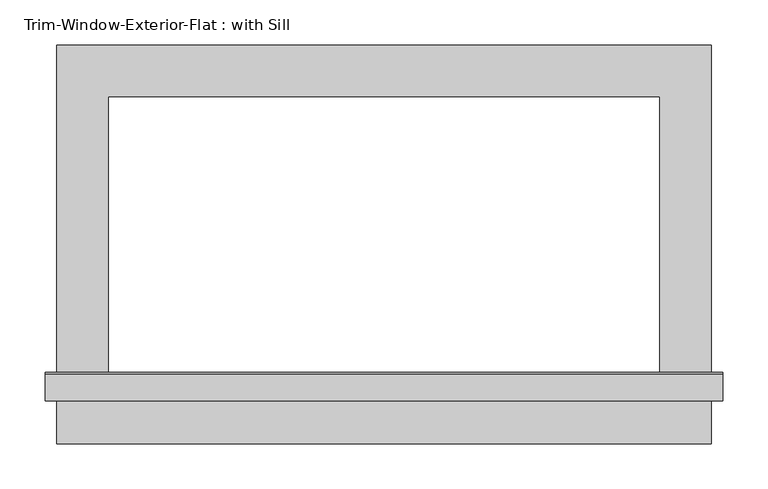
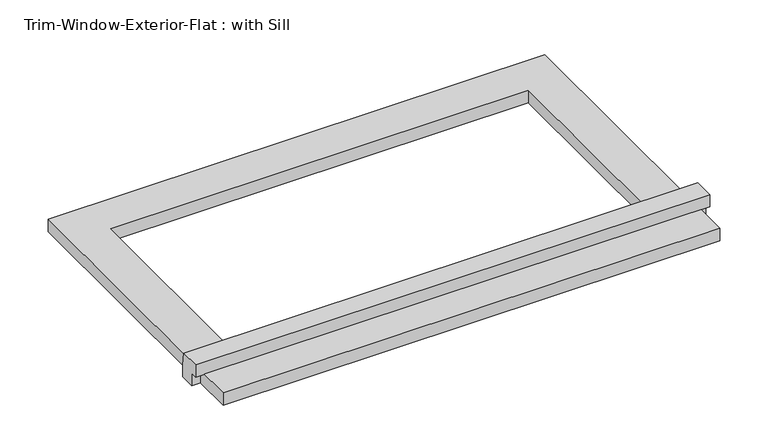
"""IFC4 building model written with IfcOpenShell, lengths in millimetres: proxy geometry, Trim-Window-Exterior-Flat : with Sill."""

from ifc_helpers import new_model, si_unit, frame, origin, origin_with_axes, place, context, project, spatial, polyline, outline, extrude, source, transform, mapped, element, save


def trim_window_exterior_flat_with_sill_281d40e2(model_context):
    return source(origin(), model_context, "Body", "SweptSolid", [
        extrude(outline(polyline([(361.95, -326.9823709), (361.95, -384.1323709), (-361.95, -384.1323709), (-361.95, -326.9823709), (361.95, -326.9823709)])), origin_with_axes(), (0.0, 0.0, 1.0), 19.05),
        extrude(outline(polyline([(-336.55, 38.1), (-307.2580645, 38.1), (-304.8, 19.05), (-304.8, 0.0), (-326.9823709, 0.0), (-326.9823709, 19.05), (-336.55, 19.05), (-336.55, 38.1)])), frame((-374.65, 0.0, 0.0), z_axis=(1.0, 0.0, 0.0), x_axis=(0.0, 1.0, 0.0)), (0.0, 0.0, 1.0), 749.3),
        extrude(outline(polyline([(-361.95, 57.15), (361.95, 57.15), (361.95, -304.8), (304.8, -304.8), (304.8, 0.0), (-304.8, 0.0), (-304.8, -304.8), (-361.95, -304.8), (-361.95, 57.15)])), origin_with_axes(), (0.0, 0.0, 1.0), 19.05),
    ])


if __name__ == "__main__":
    model = new_model("IFC4")
    model_context = context("Model", 3, world=origin())
    ifc_project = project(units=[si_unit("LENGTHUNIT", "METRE", prefix="MILLI")], contexts=[model_context])
    site = spatial("IfcSite", under=ifc_project)
    building = spatial("IfcBuilding", under=site)
    placement = place(None, origin())
    trim_window_exterior_flat_with_sill_shape = trim_window_exterior_flat_with_sill_281d40e2(model_context)
    element("IfcBuildingElementProxy", 1, Name="Trim-Window-Exterior-Flat : with Sill", ObjectType="Trim-Window-Exterior-Flat : with Sill", at=placement, inside=building, context=model_context, shape_type="MappedRepresentation", body=[
        mapped(trim_window_exterior_flat_with_sill_shape, transform((0.0, 0.0, 0.0), x_axis=(1.0, 0.0, 0.0), y_axis=(0.0, 1.0, 0.0), z_axis=(0.0, 0.0, 1.0))),
    ])
    save(model, "model.ifc")

# Revit data of these elements
# Type "Trim-Window-Exterior-Flat : with Sill"
#   Trim Width = 0' - 2 1/4"
#   Trim Thickness_Picture Frame = 0' - 1 1/4"
#   Trim Thickness_with Sill = 0' - 0 3/4"
#   Sill Thickness = 0' - 1 1/4"
#   Opening Width [instance default] = 2' - 0"
#   Opening Height [instance default] = 3' - 0"
#   Default Elevation = 4' - 0"
#   Sill = yes
#   Picture Frame = no
#   Trim Material [instance default] = none
# Element 1 (IfcBuildingElementProxy, "Trim-Window-Exterior-Flat : with Sill")
#   Opening Height = 1' - 0"
#   Trim Material = Clad - White
#   Materials on its faces: "Clad - White"
# Materials
#   "Clad - White": class "Wood", colour RGB 242 242 238, transparency 0, Cost = 0
